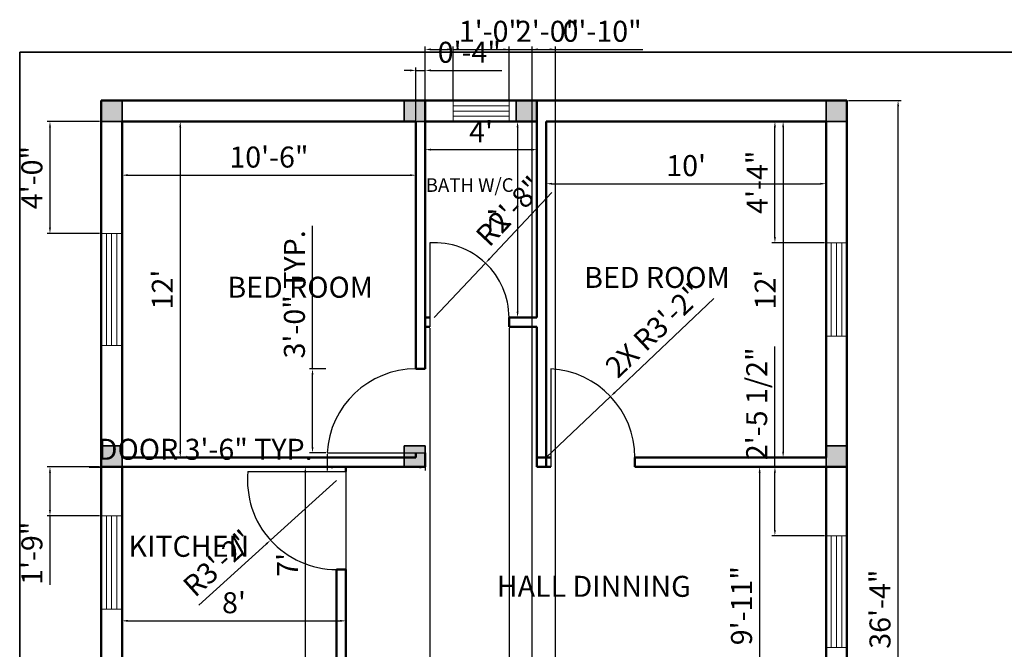
# Model space of a CAD drawing. Units: inches. Extents: x 2289 to 3796, y 1741 to 2286.
# Tile 2 of 4: x 2318 to 2741, y 1989 to 2259. Entities that reach past the tile are written whole.
import ezdxf

# ---------------------------------------------------------------- set-up
doc = ezdxf.new("R2010")
doc.units = ezdxf.units.IN
for name, color, linetype, lineweight in [('A-ANNO-DIMS', 2, 'Continuous', 18), ('A-ANNO-TTLB', 7, 'Continuous', 35), ('A-AREA-IDEN', 7, 'Continuous', 25), ('A-DOOR', 3, 'Continuous', 25), ('A-GLAZ', 4, 'Continuous', 18), ('A-WALL', 7, 'Continuous', 50), ('S-COLS', 1, 'Continuous', 35)]:
    doc.layers.add(name, color=color, linetype=linetype, lineweight=lineweight)
doc.styles.get("Standard").update_dxf_attribs({"font": 'arial.ttf'})
doc.dimstyles.new('ISO-25', dxfattribs={"dimtxt": 9, "dimasz": 2.5, "dimexe": 1.25, "dimexo": 0.625, "dimgap": 2, "dimtad": 1, "dimdec": 1, "dimlunit": 4, "dimtxsty": 'Standard', "dimcen": 2.5, "dimadec": 0, "dimazin": 0, "dimtfac": 1, "dimtdec": 1, "dimtmove": 0, "dimatfit": 3, "dimfxl": 1, "dimarcsym": 0})

# ---------------------------------------------------------------- blocks, each defined once
blk = doc.blocks.new('*D1')
at = {"layer": 'A-ANNO-DIMS', "color": 0, "lineweight": -2, "transparency": 16777216}
for p, q in [((2663.45, 2215.39), (2644.43, 2215.39)), ((2645.68, 2212.89), (2645.68, 2073.89)), ((2663.45, 2071.39), (2644.43, 2071.39))]:
    blk.add_line(p, q, dxfattribs=at)
at = {"layer": 'A-ANNO-DIMS', "color": 0, "transparency": 16777216}
for points in [[(2645.27, 2212.89), (2646.1, 2212.89), (2645.68, 2215.39)], [(2645.27, 2073.89), (2646.1, 2073.89), (2645.68, 2071.39)]]:
    blk.add_solid(points, dxfattribs=at)
at = {"layer": 'Defpoints', "color": 0, "transparency": 16777216}
for p in [(2664.08, 2215.39), (2645.68, 2071.39), (2664.08, 2071.39)]:
    blk.add_point(p, dxfattribs=at)
at = {"layer": 'A-ANNO-DIMS', "color": 0, "transparency": 16777216, "insert": (2639.16, 2143.39), "char_height": 9, "attachment_point": 5, "rotation": 90}
blk.add_mtext("12'", dxfattribs=at)
blk = doc.blocks.new('*D2')
at = {"layer": 'A-ANNO-DIMS', "color": 0, "lineweight": -2, "transparency": 16777216}
for p, q in [((2544.08, 2214.76), (2544.08, 2187.49)), ((2664.08, 2214.76), (2664.08, 2187.49)), ((2546.58, 2188.74), (2661.58, 2188.74))]:
    blk.add_line(p, q, dxfattribs=at)
at = {"layer": 'A-ANNO-DIMS', "color": 0, "transparency": 16777216}
for points in [[(2546.58, 2189.15), (2546.58, 2188.32), (2544.08, 2188.74)], [(2661.58, 2189.15), (2661.58, 2188.32), (2664.08, 2188.74)]]:
    blk.add_solid(points, dxfattribs=at)
at = {"layer": 'Defpoints', "color": 0, "transparency": 16777216}
for p in [(2544.08, 2215.39), (2664.08, 2215.39), (2664.08, 2188.74)]:
    blk.add_point(p, dxfattribs=at)
at = {"layer": 'A-ANNO-DIMS', "color": 0, "transparency": 16777216, "insert": (2604.08, 2195.33), "char_height": 9, "attachment_point": 5}
blk.add_mtext("10'", dxfattribs=at)
blk = doc.blocks.new('*D3')
at = {"layer": 'A-ANNO-DIMS', "color": 0, "lineweight": -2, "transparency": 16777216}
for p, q in [((2539.45, 2215.39), (2530.51, 2215.39)), ((2531.76, 2212.89), (2531.76, 2133.89)), ((2539.45, 2131.39), (2530.51, 2131.39))]:
    blk.add_line(p, q, dxfattribs=at)
at = {"layer": 'A-ANNO-DIMS', "color": 0, "transparency": 16777216}
for points in [[(2531.34, 2212.89), (2532.17, 2212.89), (2531.76, 2215.39)], [(2531.34, 2133.89), (2532.17, 2133.89), (2531.76, 2131.39)]]:
    blk.add_solid(points, dxfattribs=at)
at = {"layer": 'Defpoints', "color": 0, "transparency": 16777216}
for p in [(2540.08, 2215.39), (2531.76, 2131.39), (2540.08, 2131.39)]:
    blk.add_point(p, dxfattribs=at)
at = {"layer": 'A-ANNO-DIMS', "color": 0, "transparency": 16777216, "insert": (2525.26, 2173.39), "char_height": 9, "attachment_point": 5, "rotation": 90}
blk.add_mtext("7'", dxfattribs=at)
blk = doc.blocks.new('*D4')
at = {"layer": 'A-ANNO-DIMS', "color": 0, "lineweight": -2, "transparency": 16777216}
for p, q in [((2362.08, 2214.76), (2362.08, 2191.15)), ((2488.08, 2214.76), (2488.08, 2191.15)), ((2364.58, 2192.4), (2485.58, 2192.4))]:
    blk.add_line(p, q, dxfattribs=at)
at = {"layer": 'A-ANNO-DIMS', "color": 0, "transparency": 16777216}
for points in [[(2364.58, 2192.82), (2364.58, 2191.98), (2362.08, 2192.4)], [(2485.58, 2192.82), (2485.58, 2191.98), (2488.08, 2192.4)]]:
    blk.add_solid(points, dxfattribs=at)
at = {"layer": 'Defpoints', "color": 0, "transparency": 16777216}
for p in [(2362.08, 2215.39), (2488.08, 2215.39), (2488.08, 2192.4)]:
    blk.add_point(p, dxfattribs=at)
at = {"layer": 'A-ANNO-DIMS', "color": 0, "transparency": 16777216, "insert": (2425.08, 2199), "char_height": 9, "attachment_point": 5}
blk.add_mtext('10\'-6"', dxfattribs=at)
blk = doc.blocks.new('*D5')
at = {"layer": 'A-ANNO-DIMS', "color": 0, "lineweight": -2, "transparency": 16777216}
for p, q in [((2362.7, 2215.39), (2388.28, 2215.39)), ((2387.03, 2212.89), (2387.03, 2073.89)), ((2362.7, 2071.39), (2388.28, 2071.39))]:
    blk.add_line(p, q, dxfattribs=at)
at = {"layer": 'A-ANNO-DIMS', "color": 0, "transparency": 16777216}
for points in [[(2386.62, 2212.89), (2387.45, 2212.89), (2387.03, 2215.39)], [(2386.62, 2073.89), (2387.45, 2073.89), (2387.03, 2071.39)]]:
    blk.add_solid(points, dxfattribs=at)
at = {"layer": 'Defpoints', "color": 0, "transparency": 16777216}
for p in [(2362.08, 2215.39), (2362.08, 2071.39), (2387.03, 2071.39)]:
    blk.add_point(p, dxfattribs=at)
at = {"layer": 'A-ANNO-DIMS', "color": 0, "transparency": 16777216, "insert": (2380.51, 2143.39), "char_height": 9, "attachment_point": 5, "rotation": 90}
blk.add_mtext("12'", dxfattribs=at)
blk = doc.blocks.new('*D6')
at = {"layer": 'A-ANNO-DIMS', "color": 0, "lineweight": -2, "transparency": 16777216}
for p, q in [((2362.08, 2066.76), (2362.08, 2000.14)), ((2458.08, 2066.76), (2458.08, 2000.14)), ((2364.58, 2001.39), (2455.58, 2001.39))]:
    blk.add_line(p, q, dxfattribs=at)
at = {"layer": 'A-ANNO-DIMS', "color": 0, "transparency": 16777216}
for points in [[(2364.58, 2001.8), (2364.58, 2000.97), (2362.08, 2001.39)], [(2455.58, 2001.8), (2455.58, 2000.97), (2458.08, 2001.39)]]:
    blk.add_solid(points, dxfattribs=at)
at = {"layer": 'Defpoints', "color": 0, "transparency": 16777216}
for p in [(2362.08, 2067.39), (2458.08, 2067.39), (2458.08, 2001.39)]:
    blk.add_point(p, dxfattribs=at)
at = {"layer": 'A-ANNO-DIMS', "color": 0, "transparency": 16777216, "insert": (2410.08, 2007.98), "char_height": 9, "attachment_point": 5}
blk.add_mtext("8'", dxfattribs=at)
blk = doc.blocks.new('*D13')
at = {"layer": 'A-ANNO-DIMS', "color": 0, "lineweight": -2, "transparency": 16777216}
for p, q in [((2664.08, 2007.26), (2664.08, 1963)), ((2504.08, 1978.76), (2504.08, 1963)), ((2506.58, 1964.25), (2661.58, 1964.25))]:
    blk.add_line(p, q, dxfattribs=at)
at = {"layer": 'A-ANNO-DIMS', "color": 0, "transparency": 16777216}
for points in [[(2506.58, 1964.67), (2506.58, 1963.83), (2504.08, 1964.25)], [(2661.58, 1964.67), (2661.58, 1963.83), (2664.08, 1964.25)]]:
    blk.add_solid(points, dxfattribs=at)
at = {"layer": 'Defpoints', "color": 0, "transparency": 16777216}
for p in [(2664.08, 2007.89), (2504.08, 1979.39), (2664.08, 1964.25)]:
    blk.add_point(p, dxfattribs=at)
at = {"layer": 'A-ANNO-DIMS', "color": 0, "transparency": 16777216, "insert": (2584.08, 1970.85), "char_height": 9, "attachment_point": 5}
blk.add_mtext('13\'-4"', dxfattribs=at)
blk = doc.blocks.new('*D14')
at = {"layer": 'A-ANNO-DIMS', "color": 0, "lineweight": -2, "transparency": 16777216}
for p, q in [((2362.7, 2067.39), (2441.94, 2067.39)), ((2440.69, 2064.89), (2440.69, 1985.89)), ((2362.7, 1983.39), (2441.94, 1983.39))]:
    blk.add_line(p, q, dxfattribs=at)
at = {"layer": 'A-ANNO-DIMS', "color": 0, "transparency": 16777216}
for points in [[(2440.27, 2064.89), (2441.1, 2064.89), (2440.69, 2067.39)], [(2440.27, 1985.89), (2441.1, 1985.89), (2440.69, 1983.39)]]:
    blk.add_solid(points, dxfattribs=at)
at = {"layer": 'Defpoints', "color": 0, "transparency": 16777216}
for p in [(2362.08, 2067.39), (2362.08, 1983.39), (2440.69, 1983.39)]:
    blk.add_point(p, dxfattribs=at)
at = {"layer": 'A-ANNO-DIMS', "color": 0, "transparency": 16777216, "insert": (2434.19, 2025.39), "char_height": 9, "attachment_point": 5, "rotation": 90}
blk.add_mtext("7'", dxfattribs=at)
blk = doc.blocks.new('*D15')
at = {"layer": 'A-ANNO-DIMS', "color": 0, "lineweight": -2, "transparency": 16777216}
for p, q in [((2663.45, 2067.39), (2634.35, 2067.39)), ((2635.6, 2064.89), (2635.6, 1950.89)), ((2663.45, 1948.39), (2634.35, 1948.39))]:
    blk.add_line(p, q, dxfattribs=at)
at = {"layer": 'A-ANNO-DIMS', "color": 0, "transparency": 16777216}
for points in [[(2635.18, 2064.89), (2636.02, 2064.89), (2635.6, 2067.39)], [(2635.18, 1950.89), (2636.02, 1950.89), (2635.6, 1948.39)]]:
    blk.add_solid(points, dxfattribs=at)
at = {"layer": 'Defpoints', "color": 0, "transparency": 16777216}
for p in [(2664.08, 2067.39), (2635.6, 1948.39), (2664.08, 1948.39)]:
    blk.add_point(p, dxfattribs=at)
at = {"layer": 'A-ANNO-DIMS', "color": 0, "transparency": 16777216, "insert": (2629, 2007.89), "char_height": 9, "attachment_point": 5, "rotation": 90}
blk.add_mtext('9\'-11"', dxfattribs=at)
blk = doc.blocks.new('*D16')
at = {"layer": 'A-ANNO-DIMS', "color": 0, "lineweight": -2, "transparency": 16777216}
for p, q in [((2492.08, 2214.76), (2492.08, 2202.1)), ((2540.08, 2214.76), (2540.08, 2202.1)), ((2494.58, 2203.35), (2537.58, 2203.35))]:
    blk.add_line(p, q, dxfattribs=at)
at = {"layer": 'A-ANNO-DIMS', "color": 0, "transparency": 16777216}
for points in [[(2494.58, 2203.77), (2494.58, 2202.93), (2492.08, 2203.35)], [(2537.58, 2203.77), (2537.58, 2202.93), (2540.08, 2203.35)]]:
    blk.add_solid(points, dxfattribs=at)
at = {"layer": 'Defpoints', "color": 0, "transparency": 16777216}
for p in [(2492.08, 2215.39), (2540.08, 2215.39), (2540.08, 2203.35)]:
    blk.add_point(p, dxfattribs=at)
at = {"layer": 'A-ANNO-DIMS', "color": 0, "transparency": 16777216, "insert": (2516.08, 2209.85), "char_height": 9, "attachment_point": 5}
blk.add_mtext("4'", dxfattribs=at)
blk = doc.blocks.new('WIN-40IN')
for p, q in [((0, 40), (9, 40)), ((2.25, 40), (2.25, 0)), ((4.5, 40), (4.5, 0)), ((6.75, 40), (6.75, 0)), ((0, 0), (9, 0))]:
    blk.add_line(p, q)
blk = doc.blocks.new('WIN-48IN')
for p, q in [((0, 48), (9, 48)), ((2.25, 48), (2.25, 0)), ((4.5, 48), (4.5, 0)), ((6.75, 48), (6.75, 0)), ((0, 0), (9, 0))]:
    blk.add_line(p, q)
blk = doc.blocks.new('DOOR-SINGLE-38IN')
blk.add_line((0, 42), (0, 0))
blk.add_arc((-2.06, 4), 38.06, 0, 86.9037)
blk = doc.blocks.new('COL-9X9')
h = blk.add_hatch(color=256)
h.dxf.hatch_style = 1
h.paths.add_polyline_path([(0, 9), (0, 0), (9, 0), (9, 9)])
blk.add_lwpolyline([(0, 9), (9, 9), (9, 0), (0, 0)], close=True)
blk = doc.blocks.new('COL-9X9-INT')
h = blk.add_hatch(color=256)
h.dxf.hatch_style = 1
h.paths.add_polyline_path([(9, 0), (9, 9), (0, 9), (0, 0)])
blk.add_lwpolyline([(0, 9), (9, 9), (9, 0), (0, 0)], close=True)
blk = doc.blocks.new('*D29')
at = {"layer": 'A-ANNO-DIMS', "color": 0, "lineweight": -2, "transparency": 16777216}
for p, q in [((2450.08, 2072.76), (2450.08, 2065.84)), ((2492.08, 2072.76), (2492.08, 2065.84)), ((2450.08, 2067.09), (2347.95, 2067.09)), ((2489.58, 2067.09), (2452.58, 2067.09))]:
    blk.add_line(p, q, dxfattribs=at)
at = {"layer": 'A-ANNO-DIMS', "color": 0, "transparency": 16777216}
for points in [[(2452.58, 2067.5), (2452.58, 2066.67), (2450.08, 2067.09)], [(2489.58, 2067.5), (2489.58, 2066.67), (2492.08, 2067.09)]]:
    blk.add_solid(points, dxfattribs=at)
at = {"layer": 'Defpoints', "color": 0, "transparency": 16777216}
for p in [(2450.08, 2073.39), (2492.08, 2073.39), (2450.08, 2067.09)]:
    blk.add_point(p, dxfattribs=at)
at = {"layer": 'A-ANNO-DIMS', "color": 0, "transparency": 16777216, "insert": (2397.77, 2073.75), "char_height": 9, "attachment_point": 5}
blk.add_mtext('DOOR 3\'-6" TYP.', dxfattribs=at)
blk = doc.blocks.new('*D30')
at = {"layer": 'A-ANNO-DIMS', "color": 0, "lineweight": -2, "transparency": 16777216}
for p, q in [((2443.78, 2109.39), (2443.78, 2170.74)), ((2449.45, 2109.39), (2442.53, 2109.39)), ((2443.78, 2075.89), (2443.78, 2106.89)), ((2449.45, 2073.39), (2442.53, 2073.39))]:
    blk.add_line(p, q, dxfattribs=at)
at = {"layer": 'A-ANNO-DIMS', "color": 0, "transparency": 16777216}
for points in [[(2443.36, 2106.89), (2444.19, 2106.89), (2443.78, 2109.39)], [(2443.36, 2075.89), (2444.19, 2075.89), (2443.78, 2073.39)]]:
    blk.add_solid(points, dxfattribs=at)
at = {"layer": 'Defpoints', "color": 0, "transparency": 16777216}
for p in [(2443.78, 2109.39), (2450.08, 2109.39), (2450.08, 2073.39)]:
    blk.add_point(p, dxfattribs=at)
at = {"layer": 'A-ANNO-DIMS', "color": 0, "transparency": 16777216, "insert": (2437.18, 2141.31), "char_height": 9, "attachment_point": 5, "rotation": 90}
blk.add_mtext('3\'-0" TYP.', dxfattribs=at)
blk = doc.blocks.new('*D36')
at = {"layer": 'A-ANNO-DIMS', "color": 0, "lineweight": -2, "transparency": 16777216}
for p, q in [((2673.7, 2224.39), (2696.25, 2224.39)), ((2695, 1790.89), (2695, 2221.89)), ((2673.7, 1788.39), (2696.25, 1788.39))]:
    blk.add_line(p, q, dxfattribs=at)
at = {"layer": 'A-ANNO-DIMS', "color": 0, "transparency": 16777216}
for points in [[(2694.59, 2221.89), (2695.42, 2221.89), (2695, 2224.39)], [(2694.59, 1790.89), (2695.42, 1790.89), (2695, 1788.39)]]:
    blk.add_solid(points, dxfattribs=at)
at = {"layer": 'Defpoints', "color": 0, "transparency": 16777216}
for p in [(2673.08, 2224.39), (2695, 2224.39), (2673.08, 1788.39)]:
    blk.add_point(p, dxfattribs=at)
at = {"layer": 'A-ANNO-DIMS', "color": 0, "transparency": 16777216, "insert": (2688.4, 2006.39), "char_height": 9, "attachment_point": 5, "rotation": 90}
blk.add_mtext('36\'-4"', dxfattribs=at)
blk = doc.blocks.new('*D38')
at = {"layer": 'A-ANNO-DIMS', "color": 0, "lineweight": -2, "transparency": 16777216}
for p, q in [((2352.45, 2215.39), (2329.9, 2215.39)), ((2331.15, 2212.89), (2331.15, 2169.89)), ((2352.45, 2167.39), (2329.9, 2167.39))]:
    blk.add_line(p, q, dxfattribs=at)
at = {"layer": 'A-ANNO-DIMS', "color": 0, "transparency": 16777216}
for points in [[(2330.74, 2212.89), (2331.57, 2212.89), (2331.15, 2215.39)], [(2330.74, 2169.89), (2331.57, 2169.89), (2331.15, 2167.39)]]:
    blk.add_solid(points, dxfattribs=at)
at = {"layer": 'Defpoints', "color": 0, "transparency": 16777216}
for p in [(2353.08, 2215.39), (2331.15, 2167.39), (2353.08, 2167.39)]:
    blk.add_point(p, dxfattribs=at)
at = {"layer": 'A-ANNO-DIMS', "color": 0, "transparency": 16777216, "insert": (2324.56, 2191.39), "char_height": 9, "attachment_point": 5, "rotation": 90}
blk.add_mtext('4\'-0"', dxfattribs=at)
blk = doc.blocks.new('*D39')
at = {"layer": 'A-ANNO-DIMS', "color": 0, "lineweight": -2, "transparency": 16777216}
for p, q in [((2352.45, 2067.39), (2329.9, 2067.39)), ((2331.15, 2064.89), (2331.15, 2048.89)), ((2352.45, 2046.39), (2329.9, 2046.39)), ((2331.15, 2046.39), (2331.15, 2016.81))]:
    blk.add_line(p, q, dxfattribs=at)
at = {"layer": 'A-ANNO-DIMS', "color": 0, "transparency": 16777216}
for points in [[(2330.74, 2064.89), (2331.57, 2064.89), (2331.15, 2067.39)], [(2330.74, 2048.89), (2331.57, 2048.89), (2331.15, 2046.39)]]:
    blk.add_solid(points, dxfattribs=at)
at = {"layer": 'Defpoints', "color": 0, "transparency": 16777216}
for p in [(2353.08, 2067.39), (2331.15, 2046.39), (2353.08, 2046.39)]:
    blk.add_point(p, dxfattribs=at)
at = {"layer": 'A-ANNO-DIMS', "color": 0, "transparency": 16777216, "insert": (2324.56, 2030.35), "char_height": 9, "attachment_point": 5, "rotation": 90}
blk.add_mtext('1\'-9"', dxfattribs=at)
blk = doc.blocks.new('*D41')
at = {"layer": 'A-ANNO-DIMS', "color": 0, "lineweight": -2, "transparency": 16777216}
for p, q in [((2663.45, 2215.39), (2640.9, 2215.39)), ((2642.15, 2165.89), (2642.15, 2212.89)), ((2663.45, 2163.39), (2640.9, 2163.39))]:
    blk.add_line(p, q, dxfattribs=at)
at = {"layer": 'A-ANNO-DIMS', "color": 0, "transparency": 16777216}
for points in [[(2641.74, 2212.89), (2642.57, 2212.89), (2642.15, 2215.39)], [(2641.74, 2165.89), (2642.57, 2165.89), (2642.15, 2163.39)]]:
    blk.add_solid(points, dxfattribs=at)
at = {"layer": 'Defpoints', "color": 0, "transparency": 16777216}
for p in [(2642.15, 2215.39), (2664.08, 2215.39), (2664.08, 2163.39)]:
    blk.add_point(p, dxfattribs=at)
at = {"layer": 'A-ANNO-DIMS', "color": 0, "transparency": 16777216, "insert": (2635.65, 2189.39), "char_height": 9, "attachment_point": 5, "rotation": 90}
blk.add_mtext('4\'-4"', dxfattribs=at)
blk = doc.blocks.new('*D42')
at = {"layer": 'A-ANNO-DIMS', "color": 0, "lineweight": -2, "transparency": 16777216}
for p, q in [((2642.15, 2067.39), (2642.15, 2118.93)), ((2663.45, 2067.39), (2640.9, 2067.39)), ((2642.15, 2040.39), (2642.15, 2064.89)), ((2663.45, 2037.89), (2640.9, 2037.89))]:
    blk.add_line(p, q, dxfattribs=at)
at = {"layer": 'A-ANNO-DIMS', "color": 0, "transparency": 16777216}
for points in [[(2641.74, 2064.89), (2642.57, 2064.89), (2642.15, 2067.39)], [(2641.74, 2040.39), (2642.57, 2040.39), (2642.15, 2037.89)]]:
    blk.add_solid(points, dxfattribs=at)
at = {"layer": 'Defpoints', "color": 0, "transparency": 16777216}
for p in [(2642.15, 2067.39), (2664.08, 2067.39), (2664.08, 2037.89)]:
    blk.add_point(p, dxfattribs=at)
at = {"layer": 'A-ANNO-DIMS', "color": 0, "transparency": 16777216, "insert": (2635.5, 2094.41), "char_height": 9, "attachment_point": 5, "rotation": 90}
blk.add_mtext('2\'-5 1/2"', dxfattribs=at)
blk = doc.blocks.new('*D44')
at = {"layer": 'A-ANNO-DIMS', "color": 0, "lineweight": -2, "transparency": 16777216}
for p, q in [((2492.08, 2225.01), (2492.08, 2247.56)), ((2504.08, 2225.01), (2504.08, 2247.56)), ((2494.58, 2246.31), (2501.58, 2246.31)), ((2504.08, 2246.31), (2533.65, 2246.31))]:
    blk.add_line(p, q, dxfattribs=at)
at = {"layer": 'A-ANNO-DIMS', "color": 0, "transparency": 16777216}
for points in [[(2494.58, 2246.73), (2494.58, 2245.89), (2492.08, 2246.31)], [(2501.58, 2246.73), (2501.58, 2245.89), (2504.08, 2246.31)]]:
    blk.add_solid(points, dxfattribs=at)
at = {"layer": 'Defpoints', "color": 0, "transparency": 16777216}
for p in [(2504.08, 2246.31), (2492.08, 2224.39), (2504.08, 2224.39)]:
    blk.add_point(p, dxfattribs=at)
at = {"layer": 'A-ANNO-DIMS', "color": 0, "transparency": 16777216, "insert": (2520.12, 2252.91), "char_height": 9, "attachment_point": 5}
blk.add_mtext('1\'-0"', dxfattribs=at)
blk = doc.blocks.new('*D45')
at = {"layer": 'A-ANNO-DIMS', "color": 0, "lineweight": -2, "transparency": 16777216}
for p, q in [((2504.08, 2225.01), (2504.08, 2247.56)), ((2528.08, 2225.01), (2528.08, 2247.56)), ((2506.58, 2246.31), (2525.58, 2246.31)), ((2528.08, 2246.31), (2558.65, 2246.31))]:
    blk.add_line(p, q, dxfattribs=at)
at = {"layer": 'A-ANNO-DIMS', "color": 0, "transparency": 16777216}
for points in [[(2506.58, 2246.73), (2506.58, 2245.89), (2504.08, 2246.31)], [(2525.58, 2246.73), (2525.58, 2245.89), (2528.08, 2246.31)]]:
    blk.add_solid(points, dxfattribs=at)
at = {"layer": 'Defpoints', "color": 0, "transparency": 16777216}
for p in [(2528.08, 2246.31), (2504.08, 2224.39), (2528.08, 2224.39)]:
    blk.add_point(p, dxfattribs=at)
at = {"layer": 'A-ANNO-DIMS', "color": 0, "transparency": 16777216, "insert": (2544.62, 2252.91), "char_height": 9, "attachment_point": 5}
blk.add_mtext('2\'-0"', dxfattribs=at)
blk = doc.blocks.new('*D46')
at = {"layer": 'A-ANNO-DIMS', "color": 0, "lineweight": -2, "transparency": 16777216}
for p, q in [((2494.08, 2126.76), (2494.08, 1765.21)), ((2528.08, 2126.76), (2528.08, 1765.21)), ((2496.58, 1766.46), (2525.58, 1766.46)), ((2528.08, 1766.46), (2565.65, 1766.46))]:
    blk.add_line(p, q, dxfattribs=at)
at = {"layer": 'A-ANNO-DIMS', "color": 0, "transparency": 16777216}
for points in [[(2496.58, 1766.88), (2496.58, 1766.04), (2494.08, 1766.46)], [(2525.58, 1766.88), (2525.58, 1766.04), (2528.08, 1766.46)]]:
    blk.add_solid(points, dxfattribs=at)
at = {"layer": 'Defpoints', "color": 0, "transparency": 16777216}
for p in [(2494.08, 2127.39), (2528.08, 2127.39), (2528.08, 1766.46)]:
    blk.add_point(p, dxfattribs=at)
at = {"layer": 'A-ANNO-DIMS', "color": 0, "transparency": 16777216, "insert": (2548.11, 1773.06), "char_height": 9, "attachment_point": 5}
blk.add_mtext('2\'-10"', dxfattribs=at)
blk = doc.blocks.new('*D47')
at = {"layer": 'A-ANNO-DIMS', "color": 0, "lineweight": -2, "transparency": 16777216}
for p, q in [((2485.58, 2237.31), (2483.08, 2237.31)), ((2488.08, 2216.01), (2488.08, 2238.56)), ((2488.08, 2237.31), (2492.08, 2237.31)), ((2492.08, 2216.01), (2492.08, 2238.56)), ((2494.58, 2237.31), (2525, 2237.31))]:
    blk.add_line(p, q, dxfattribs=at)
at = {"layer": 'A-ANNO-DIMS', "color": 0, "transparency": 16777216}
for points in [[(2485.58, 2237.73), (2485.58, 2236.89), (2488.08, 2237.31)], [(2494.58, 2237.73), (2494.58, 2236.89), (2492.08, 2237.31)]]:
    blk.add_solid(points, dxfattribs=at)
at = {"layer": 'Defpoints', "color": 0, "transparency": 16777216}
for p in [(2492.08, 2237.31), (2488.08, 2215.39), (2492.08, 2215.39)]:
    blk.add_point(p, dxfattribs=at)
at = {"layer": 'A-ANNO-DIMS', "color": 0, "transparency": 16777216, "insert": (2511.04, 2243.91), "char_height": 9, "attachment_point": 5}
blk.add_mtext('0\'-4"', dxfattribs=at)
blk = doc.blocks.new('*D48')
at = {"layer": 'A-ANNO-DIMS', "color": 0, "lineweight": -2, "transparency": 16777216}
for p, q in [((2538.08, 1945.01), (2538.08, 2247.56)), ((2548.08, 1945.01), (2548.08, 2247.56)), ((2540.58, 2246.31), (2545.58, 2246.31)), ((2548.08, 2246.31), (2585.49, 2246.31))]:
    blk.add_line(p, q, dxfattribs=at)
at = {"layer": 'A-ANNO-DIMS', "color": 0, "transparency": 16777216}
for points in [[(2540.58, 2246.73), (2540.58, 2245.89), (2538.08, 2246.31)], [(2545.58, 2246.73), (2545.58, 2245.89), (2548.08, 2246.31)]]:
    blk.add_solid(points, dxfattribs=at)
at = {"layer": 'Defpoints', "color": 0, "transparency": 16777216}
for p in [(2548.08, 2246.31), (2538.08, 1944.39), (2548.08, 1944.39)]:
    blk.add_point(p, dxfattribs=at)
at = {"layer": 'A-ANNO-DIMS', "color": 0, "transparency": 16777216, "insert": (2568.04, 2252.91), "char_height": 9, "attachment_point": 5}
blk.add_mtext('0\'-10"', dxfattribs=at)
blk = doc.blocks.new('*D75')
at = {"layer": 'A-ANNO-DIMS', "color": 0, "lineweight": -2, "transparency": 16777216}
for p, q in [((2454.08, 2061.58), (2425.76, 2035.95)), ((2394.96, 2008.09), (2423.9, 2034.28))]:
    blk.add_line(p, q, dxfattribs=at)
at = {"layer": 'A-ANNO-DIMS', "color": 0, "transparency": 16777216}
blk.add_solid([(2423.62, 2034.59), (2424.18, 2033.97), (2425.76, 2035.95)], dxfattribs=at)
at = {"layer": 'Defpoints', "color": 0, "transparency": 16777216}
for p in [(2454.08, 2061.58), (2425.76, 2035.95)]:
    blk.add_point(p, dxfattribs=at)
at = {"layer": 'A-ANNO-DIMS', "color": 0, "transparency": 16777216, "insert": (2404.08, 2025.24), "char_height": 9, "attachment_point": 5, "rotation": 42.1378}
blk.add_mtext('R3\'-2"', dxfattribs=at)
blk = doc.blocks.new('*D76')
at = {"layer": 'A-ANNO-DIMS', "color": 0, "lineweight": -2, "transparency": 16777216}
for p, q in [((2546.46, 2184.98), (2519.7, 2156.55)), ((2496.02, 2131.39), (2517.99, 2154.73))]:
    blk.add_line(p, q, dxfattribs=at)
at = {"layer": 'A-ANNO-DIMS', "color": 0, "transparency": 16777216}
blk.add_solid([(2519.4, 2156.84), (2520.01, 2156.27), (2517.99, 2154.73)], dxfattribs=at)
at = {"layer": 'Defpoints', "color": 0, "transparency": 16777216}
for p in [(2517.99, 2154.73), (2496.02, 2131.39)]:
    blk.add_point(p, dxfattribs=at)
at = {"layer": 'A-ANNO-DIMS', "color": 0, "transparency": 16777216, "insert": (2529.14, 2176.2), "char_height": 9, "attachment_point": 5, "rotation": 46.7361}
blk.add_mtext('R2\'-8"', dxfattribs=at)
blk = doc.blocks.new('*D77')
at = {"layer": 'A-ANNO-DIMS', "color": 0, "lineweight": -2, "transparency": 16777216}
for p, q in [((2615.95, 2139.53), (2573.46, 2099.28)), ((2544.02, 2071.39), (2571.65, 2097.56))]:
    blk.add_line(p, q, dxfattribs=at)
at = {"layer": 'A-ANNO-DIMS', "color": 0, "transparency": 16777216}
blk.add_solid([(2573.18, 2099.58), (2573.75, 2098.98), (2571.65, 2097.56)], dxfattribs=at)
at = {"layer": 'Defpoints', "color": 0, "transparency": 16777216}
for p in [(2571.65, 2097.56), (2544.02, 2071.39)]:
    blk.add_point(p, dxfattribs=at)
at = {"layer": 'A-ANNO-DIMS', "color": 0, "transparency": 16777216, "insert": (2591.08, 2125.05), "char_height": 9, "attachment_point": 5, "rotation": 43.4516}
blk.add_mtext('2X R3\'-2"', dxfattribs=at)

msp = doc.modelspace()

# ---------------------------------------------------------------- linework, layer by layer
at = {"layer": 'A-ANNO-TTLB'}
msp.add_lwpolyline([(2318.16, 2245.19), (3750.19, 2245.19), (3750.19, 1741.69), (2318.16, 1741.69)], close=True, dxfattribs=at)
at = {"layer": 'A-DOOR'}
for p, q in [((2494.08, 2163.39), (2494.08, 2127.39)), ((2416.08, 2065.39), (2458.08, 2065.39))]:
    msp.add_line(p, q, dxfattribs=at)
for centre, radius, start, end in [((2496.02, 2131.39), 32.06, 360, 93.4714), ((2454.08, 2061.58), 38.19, 174.2752, 270)]:
    msp.add_arc(centre, radius, start, end, dxfattribs=at)
at = {"layer": 'A-GLAZ'}
for p, q in [((2504.08, 2224.39), (2504.08, 2215.39)), ((2504.08, 2222.14), (2528.08, 2222.14)), ((2528.08, 2224.39), (2528.08, 2215.39)), ((2504.08, 2219.89), (2528.08, 2219.89)), ((2504.08, 2217.64), (2528.08, 2217.64)), ((2355.33, 2167.39), (2355.33, 2119.39)), ((2357.58, 2167.39), (2357.58, 2119.39)), ((2355.33, 2046.39), (2355.33, 2006.39)), ((2357.58, 2046.39), (2357.58, 2006.39))]:
    msp.add_line(p, q, dxfattribs=at)
at = {"layer": 'A-WALL'}
for p, q in [((2353.08, 2224.39), (2673.08, 2224.39)), ((2353.08, 2224.39), (2353.08, 1808.39)), ((2492.08, 2224.39), (2492.08, 2109.39)), ((2540.08, 2224.39), (2540.08, 2131.39)), ((2673.08, 2224.39), (2673.08, 1808.39)), ((2362.08, 2215.39), (2488.08, 2215.39)), ((2362.08, 2215.39), (2362.08, 2071.39)), ((2488.08, 2215.39), (2488.08, 2109.39)), ((2492.08, 2215.39), (2540.08, 2215.39)), ((2544.08, 2215.39), (2544.08, 2067.39)), ((2544.08, 2215.39), (2664.08, 2215.39)), ((2664.08, 2215.39), (2664.08, 2071.39)), ((2492.08, 2131.39), (2494.08, 2131.39)), ((2528.08, 2131.39), (2528.08, 2127.39)), ((2528.08, 2131.39), (2540.08, 2131.39)), ((2492.08, 2127.39), (2494.08, 2127.39)), ((2528.08, 2127.39), (2540.08, 2127.39)), ((2540.08, 2127.39), (2540.08, 2067.39)), ((2488.08, 2109.39), (2492.08, 2109.39)), ((2362.08, 2071.39), (2488.08, 2071.39)), ((2488.08, 2073.39), (2488.08, 2071.39)), ((2492.08, 2073.39), (2492.08, 2067.39)), ((2540.08, 2071.39), (2546.08, 2071.39)), ((2582.08, 2071.39), (2664.08, 2071.39)), ((2582.08, 2071.39), (2582.08, 2067.39)), ((2353.08, 2067.39), (2492.08, 2067.39)), ((2362.08, 2067.39), (2362.08, 1983.39)), ((2458.08, 2067.39), (2458.08, 2065.39)), ((2540.08, 2067.39), (2546.08, 2067.39)), ((2582.08, 2067.39), (2673.08, 2067.39)), ((2664.08, 2067.39), (2664.08, 1948.39)), ((2454.08, 2023.39), (2458.08, 2023.39)), ((2454.08, 2023.39), (2454.08, 1983.39)), ((2458.08, 2023.39), (2458.08, 1979.39))]:
    msp.add_line(p, q, dxfattribs=at)

# ---------------------------------------------------------------- block references
at = {"layer": 'A-DOOR', "rotation": 90.00000000000108}
msp.add_blockref('DOOR-SINGLE-38IN', (2492.08, 2073.39), dxfattribs=at)
at = {"layer": 'A-DOOR'}
msp.add_blockref('DOOR-SINGLE-38IN', (2546.08, 2067.39), dxfattribs=at)
at = {"layer": 'A-GLAZ', "rotation": 180}
for name, p in [('WIN-48IN', (2362.08, 2167.39)), ('WIN-40IN', (2362.08, 2046.39))]:
    msp.add_blockref(name, p, dxfattribs=at)
at = {"layer": 'A-GLAZ'}
for name, p in [('WIN-40IN', (2664.08, 2123.39)), ('WIN-48IN', (2664.08, 1989.89))]:
    msp.add_blockref(name, p, dxfattribs=at)
at = {"layer": 'S-COLS'}
for name, p in [('COL-9X9', (2353.08, 2215.39)), ('COL-9X9', (2483.08, 2215.39)), ('COL-9X9', (2531.08, 2215.39)), ('COL-9X9', (2664.08, 2215.39)), ('COL-9X9', (2353.08, 2067.39)), ('COL-9X9-INT', (2483.08, 2067.39)), ('COL-9X9', (2664.08, 2067.39))]:
    msp.add_blockref(name, p, dxfattribs=at)

# ---------------------------------------------------------------- texts
at = {"layer": 'A-AREA-IDEN'}
for s, height, p in [('BATH W/C', 5.848, (2492.36, 2185.25)), ('BED ROOM', 9, (2560.32, 2144.08)), ('BED ROOM', 9, (2407.26, 2139.88)), (' KITCHEN', 9, (2362.1, 2028.83)), ('HALL DINNING', 9, (2522.86, 2011.68))]:
    msp.add_text(s, height=height, dxfattribs=at).set_placement(p)

# ---------------------------------------------------------------- dimensions: what is measured, and where the dimension line sits
at = {"layer": 'A-ANNO-DIMS'}
for base, p1, p2, override, picture, middle in [((2504.08, 2246.31), (2492.08, 2224.39), (2504.08, 2224.39), {"dimdec": 1, "dimlfac": 1, "dimrnd": 0, "dimzin": 1, "dimdsep": 46, "dimlunit": 4, "dimfrac": 2}, '*D44', (2520.12, 2252.91)), ((2528.08, 2246.31), (2504.08, 2224.39), (2528.08, 2224.39), {"dimdec": 1, "dimlfac": 1, "dimrnd": 0, "dimzin": 1, "dimdsep": 46, "dimlunit": 4, "dimfrac": 2}, '*D45', (2544.62, 2252.91)), ((2548.08, 2246.31), (2538.08, 1944.39), (2548.08, 1944.39), {"dimdec": 1, "dimlfac": 1, "dimrnd": 0, "dimzin": 1, "dimdsep": 46, "dimlunit": 4, "dimfrac": 2}, '*D48', (2568.04, 2252.91)), ((2488.08, 2192.4), (2362.08, 2215.39), (2488.08, 2215.39), {"dimclrd": 0, "dimclre": 0, "dimclrt": 0}, '*D4', (2425.08, 2199)), ((2540.08, 2203.35), (2492.08, 2215.39), (2540.08, 2215.39), {"dimclrd": 0, "dimclre": 0, "dimclrt": 0}, '*D16', (2516.08, 2209.85)), ((2664.08, 2188.74), (2544.08, 2215.39), (2664.08, 2215.39), {"dimclrd": 0, "dimclre": 0, "dimclrt": 0}, '*D2', (2604.08, 2195.33)), ((2528.08, 1766.46), (2494.08, 2127.39), (2528.08, 2127.39), {"dimdec": 1, "dimlfac": 1, "dimrnd": 0, "dimzin": 1, "dimdsep": 46, "dimlunit": 4, "dimfrac": 2}, '*D46', (2548.11, 1773.06)), ((2458.08, 2001.39), (2362.08, 2067.39), (2458.08, 2067.39), {"dimclrd": 0, "dimclre": 0, "dimclrt": 0}, '*D6', (2410.08, 2007.98)), ((2664.08, 1964.25), (2504.08, 1979.39), (2664.08, 2007.89), {"dimclrd": 0, "dimclre": 0, "dimclrt": 0}, '*D13', (2584.08, 1970.85))]:
    dim = msp.add_linear_dim(base=base, p1=p1, p2=p2, dimstyle='ISO-25', override=override, dxfattribs=at)
    dim.commit()
    dim.dimension.update_dxf_attribs({"geometry": picture, "text_midpoint": middle})
for base, p1, p2, angle, override, picture, middle in [((2492.08, 2237.31), (2488.08, 2215.39), (2492.08, 2215.39), 0, {"dimdec": 1, "dimlfac": 1, "dimrnd": 0, "dimzin": 1, "dimdsep": 46, "dimlunit": 4, "dimfrac": 2}, '*D47', (2511.04, 2243.91)), ((2695, 2224.39), (2673.08, 1788.39), (2673.08, 2224.39), 90, {"dimdec": 1, "dimlfac": 1, "dimrnd": 0, "dimzin": 1, "dimdsep": 46, "dimlunit": 4, "dimfrac": 2}, '*D36', (2688.4, 2006.39)), ((2331.15, 2167.39), (2353.08, 2215.39), (2353.08, 2167.39), 90, {"dimdec": 1, "dimlfac": 1, "dimrnd": 0, "dimzin": 1, "dimdsep": 46, "dimlunit": 4, "dimfrac": 2}, '*D38', (2324.56, 2191.39)), ((2387.03, 2071.39), (2362.08, 2215.39), (2362.08, 2071.39), 90, {"dimclrd": 0, "dimclre": 0, "dimclrt": 0}, '*D5', (2380.51, 2143.39)), ((2531.76, 2131.39), (2540.08, 2215.39), (2540.08, 2131.39), 90, {"dimclrd": 0, "dimclre": 0, "dimclrt": 0}, '*D3', (2525.26, 2173.39)), ((2642.15, 2215.39), (2664.08, 2163.39), (2664.08, 2215.39), 90, {"dimdec": 1, "dimlfac": 1, "dimrnd": 0, "dimzin": 1, "dimdsep": 46, "dimlunit": 4, "dimfrac": 2}, '*D41', (2635.65, 2189.39)), ((2645.68, 2071.39), (2664.08, 2215.39), (2664.08, 2071.39), 90, {"dimclrd": 0, "dimclre": 0, "dimclrt": 0}, '*D1', (2639.16, 2143.39)), ((2642.15, 2067.39), (2664.08, 2037.89), (2664.08, 2067.39), 90, {"dimdec": 1, "dimlfac": 1, "dimrnd": 0, "dimzin": 1, "dimdsep": 46, "dimlunit": 4, "dimfrac": 2}, '*D42', (2635.5, 2094.41)), ((2331.15, 2046.39), (2353.08, 2067.39), (2353.08, 2046.39), 90, {"dimdec": 1, "dimlfac": 1, "dimrnd": 0, "dimzin": 1, "dimdsep": 46, "dimlunit": 4, "dimfrac": 2}, '*D39', (2324.56, 2030.35)), ((2440.69, 1983.39), (2362.08, 2067.39), (2362.08, 1983.39), 90, {"dimclrd": 0, "dimclre": 0, "dimclrt": 0}, '*D14', (2434.19, 2025.39)), ((2635.6, 1948.39), (2664.08, 2067.39), (2664.08, 1948.39), 90, {"dimclrd": 0, "dimclre": 0, "dimclrt": 0}, '*D15', (2629, 2007.89))]:
    dim = msp.add_linear_dim(base=base, p1=p1, p2=p2, angle=angle, dimstyle='ISO-25', override=override, dxfattribs=at)
    dim.commit()
    dim.dimension.update_dxf_attribs({"geometry": picture, "text_midpoint": middle})
for center, mpoint, picture, middle in [((2496.02, 2131.39), (2517.99, 2154.73), '*D76', (2529.14, 2176.2)), ((2454.08, 2061.58), (2425.76, 2035.95), '*D75', (2404.08, 2025.24))]:
    dim = msp.add_radius_dim(center=center, mpoint=mpoint, dimstyle='ISO-25', override={"dimdec": 1, "dimlfac": 1, "dimrnd": 0, "dimzin": 1, "dimdsep": 46, "dimlunit": 4, "dimfrac": 2}, dxfattribs=at)
    dim.commit()
    dim.dimension.update_dxf_attribs({"geometry": picture, "text_midpoint": middle})
for base, p1, p2, angle, text, picture, middle in [((2443.78, 2109.39), (2450.08, 2073.39), (2450.08, 2109.39), 90, '<> TYP.', '*D30', (2437.18, 2141.31)), ((2450.08, 2067.09), (2492.08, 2073.39), (2450.08, 2073.39), 180, 'DOOR <> TYP.', '*D29', (2397.77, 2073.75))]:
    dim = msp.add_linear_dim(base=base, p1=p1, p2=p2, angle=angle, text=text, dimstyle='ISO-25', override={"dimdec": 1, "dimlfac": 1, "dimrnd": 0, "dimzin": 1, "dimdsep": 46, "dimlunit": 4, "dimfrac": 2}, dxfattribs=at)
    dim.commit()
    dim.dimension.update_dxf_attribs({"geometry": picture, "text_midpoint": middle})
dim = msp.add_radius_dim(center=(2544.02, 2071.39), mpoint=(2571.65, 2097.56), text='2X <>', dimstyle='ISO-25', override={"dimdec": 1, "dimlfac": 1, "dimrnd": 0, "dimzin": 1, "dimdsep": 46, "dimlunit": 4, "dimfrac": 2}, dxfattribs=at)
dim.commit()
dim.dimension.update_dxf_attribs({"geometry": '*D77', "text_midpoint": (2591.08, 2125.05)})

doc.saveas('drawing.dxf')
